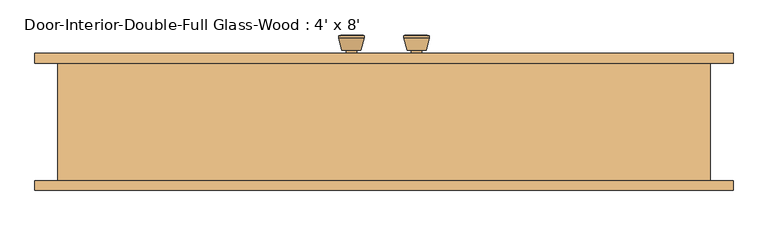
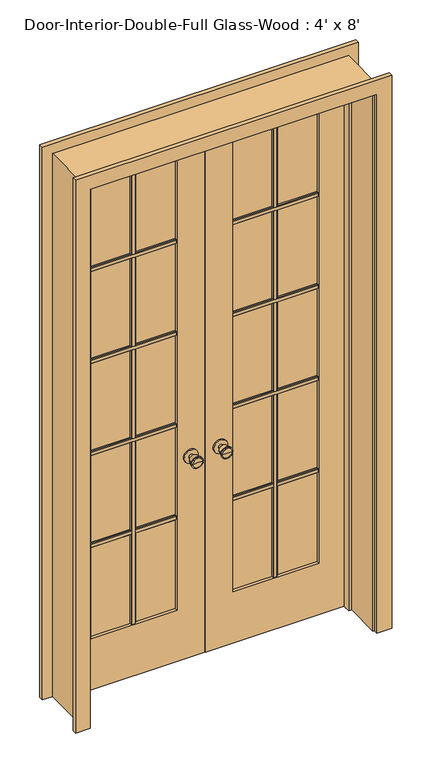
"""IFC4 building model written with IfcOpenShell, lengths in millimetres: door geometry, Door-Interior-Double-Full Glass-Wood : 4' x 8'."""

from ifc_helpers import new_model, si_unit, point, frame, frame_2d, origin, place, context, project, spatial, polyline, circle_curve, trimmed, segment, composite_curve, outline, extrude, faceted_brep, source, transform, mapped, element, save
from ifc_brep_helpers import plane_surface, cylinder_surface, revolved_surface, advanced_brep


def door_interior_double_full_glass_wood_4_x_8_0c92ad92(model_context):
    return source(origin(), model_context, "Body", "SolidModel", [
        advanced_brep(
        [(-63.5, 117.125, 914.4), (-73.5, 117.125, 914.4), (-53.5, 117.125, 914.4), (-83.9758676, 166.125, 914.4), (-63.5, 166.125, 914.4), (-43.0241324, 166.125, 914.4), (-88.5, 164.2971319, 914.4), (-38.5, 164.2971319, 914.4), (-88.5, 160.8334537, 914.4), (-38.5, 160.8334537, 914.4), (-82.136236, 136.125, 914.4), (-44.863764, 136.125, 914.4), (-73.5, 136.125, 914.4), (-53.5, 136.125, 914.4)],
        [
            (0, 1),
            (1, 2, circle_curve(frame((-63.5, 117.125, 914.4), z_axis=(0.0, -1.0, 0.0), x_axis=(1.0, 0.0, 0.0)), 10.0)),
            (2, 0),
            (2, 1, circle_curve(frame((-63.5, 117.125, 914.4), z_axis=(0.0, -1.0, 0.0), x_axis=(1.0, 0.0, 0.0)), 10.0)),
            (3, 4),
            (4, 5),
            (5, 3, circle_curve(frame((-63.5, 166.125, 914.4), z_axis=(0.0, 1.0, 0.0), x_axis=(1.0, 0.0, 0.0)), 20.4758676)),
            (3, 5, circle_curve(frame((-63.5, 166.125, 914.4), z_axis=(0.0, 1.0, 0.0), x_axis=(1.0, 0.0, 0.0)), 20.4758676)),
            (6, 3),
            (5, 7),
            (7, 6, circle_curve(frame((-63.5, 164.2971319, 914.4), z_axis=(0.0, 1.0, 0.0), x_axis=(1.0, 0.0, 0.0)), 25.0)),
            (6, 7, circle_curve(frame((-63.5, 164.2971319, 914.4), z_axis=(0.0, 1.0, 0.0), x_axis=(1.0, 0.0, 0.0)), 25.0)),
            (8, 6),
            (7, 9),
            (9, 8, circle_curve(frame((-63.5, 160.8334537, 914.4), z_axis=(0.0, 1.0, 0.0), x_axis=(1.0, 0.0, 0.0)), 25.0)),
            (8, 9, circle_curve(frame((-63.5, 160.8334537, 914.4), z_axis=(0.0, 1.0, 0.0), x_axis=(1.0, 0.0, 0.0)), 25.0)),
            (10, 8),
            (9, 11),
            (11, 10, circle_curve(frame((-63.5, 136.125, 914.4), z_axis=(0.0, 1.0, 0.0), x_axis=(1.0, 0.0, 0.0)), 18.636236)),
            (10, 11, circle_curve(frame((-63.5, 136.125, 914.4), z_axis=(0.0, 1.0, 0.0), x_axis=(1.0, 0.0, 0.0)), 18.636236)),
            (12, 10),
            (11, 13),
            (13, 12, circle_curve(frame((-63.5, 136.125, 914.4), z_axis=(0.0, 1.0, 0.0), x_axis=(1.0, 0.0, 0.0)), 10.0)),
            (12, 13, circle_curve(frame((-63.5, 136.125, 914.4), z_axis=(0.0, 1.0, 0.0), x_axis=(1.0, 0.0, 0.0)), 10.0)),
            (1, 12),
            (13, 2),
        ],
        [
            plane_surface(frame((-63.5, 117.125, 914.4), z_axis=(0.0, -1.0, 0.0), x_axis=(1.0, 0.0, 0.0))),
            plane_surface(frame((-63.5, 166.125, 914.4), z_axis=(0.0, 1.0, 0.0), x_axis=(1.0, 0.0, 0.0))),
            revolved_surface(polyline([(-43.0241324, 166.125, 914.4), (-38.5, 164.2971319, 914.4)]), (-63.5, 117.125, 914.4), (0.0, -1.0, 0.0)),
            cylinder_surface(frame((-63.5, 117.125, 914.4), z_axis=(0.0, -1.0, 0.0), x_axis=(1.0, 0.0, 0.0)), 25.0),
            revolved_surface(polyline([(-38.5, 160.8334537, 914.4), (-44.863764, 136.125, 914.4)]), (-63.5, 117.125, 914.4), (0.0, -1.0, 0.0)),
            plane_surface(frame((-63.5, 136.125, 914.4), z_axis=(0.0, -1.0, 0.0), x_axis=(1.0, 0.0, 0.0))),
            cylinder_surface(frame((-63.5, 117.125, 914.4), z_axis=(0.0, -1.0, 0.0), x_axis=(1.0, 0.0, 0.0)), 10.0),
        ],
        [
            (0, [[1, 2, 3]]),
            (0, [[-3, 4, -1]]),
            (1, [[5, 6, 7]]),
            (1, [[-6, -5, 8]]),
            (2, [[9, -7, 10, 11]]),
            (2, [[-10, -8, -9, 12]]),
            (3, [[13, -11, 14, 15]]),
            (3, [[-14, -12, -13, 16]]),
            (4, [[17, -15, 18, 19]]),
            (4, [[-18, -16, -17, 20]]),
            (5, [[21, -19, 22, 23]]),
            (5, [[-22, -20, -21, 24]]),
            (6, [[25, -23, 26, -2]]),
            (6, [[-26, -24, -25, -4]]),
        ],
    ),
        extrude(outline(composite_curve([segment(trimmed(circle_curve(frame_2d((914.4, -63.5)), 30.0), [point((914.4, -33.5))], [point((914.4, -93.5))], False, "CARTESIAN"), True, "CONTINUOUS"), segment(trimmed(circle_curve(frame_2d((914.4, -63.5)), 30.0), [point((914.4, -93.5))], [point((914.4, -33.5))], False, "CARTESIAN"), True, "CONTINUOUS")], self_intersect=False)), frame((0.0, 111.125, 0.0), z_axis=(0.0, 1.0, 0.0), x_axis=(0.0, 0.0, 1.0)), (0.0, 0.0, 1.0), 6.0),
        advanced_brep(
        [(-63.5, 70.2, 914.4), (-53.5, 70.2, 914.4), (-73.5, 70.2, 914.4), (-83.9758676, 21.2, 914.4), (-43.0241324, 21.2, 914.4), (-63.5, 21.2, 914.4), (-88.5, 23.0278681, 914.4), (-38.5, 23.0278681, 914.4), (-88.5, 26.4915463, 914.4), (-38.5, 26.4915463, 914.4), (-82.136236, 51.2, 914.4), (-44.863764, 51.2, 914.4), (-73.5, 51.2, 914.4), (-53.5, 51.2, 914.4)],
        [
            (0, 1),
            (1, 2, circle_curve(frame((-63.5, 70.2, 914.4), z_axis=(0.0, 1.0, 0.0), x_axis=(1.0, 0.0, 0.0)), 10.0)),
            (2, 0),
            (2, 1, circle_curve(frame((-63.5, 70.2, 914.4), z_axis=(0.0, 1.0, 0.0), x_axis=(1.0, 0.0, 0.0)), 10.0)),
            (3, 4, circle_curve(frame((-63.5, 21.2, 914.4), z_axis=(0.0, -1.0, 0.0), x_axis=(1.0, 0.0, 0.0)), 20.4758676)),
            (4, 5),
            (5, 3),
            (4, 3, circle_curve(frame((-63.5, 21.2, 914.4), z_axis=(0.0, -1.0, 0.0), x_axis=(1.0, 0.0, 0.0)), 20.4758676)),
            (6, 7, circle_curve(frame((-63.5, 23.0278681, 914.4), z_axis=(0.0, -1.0, 0.0), x_axis=(1.0, 0.0, 0.0)), 25.0)),
            (7, 4),
            (3, 6),
            (7, 6, circle_curve(frame((-63.5, 23.0278681, 914.4), z_axis=(0.0, -1.0, 0.0), x_axis=(1.0, 0.0, 0.0)), 25.0)),
            (8, 9, circle_curve(frame((-63.5, 26.4915463, 914.4), z_axis=(0.0, -1.0, 0.0), x_axis=(1.0, 0.0, 0.0)), 25.0)),
            (9, 7),
            (6, 8),
            (9, 8, circle_curve(frame((-63.5, 26.4915463, 914.4), z_axis=(0.0, -1.0, 0.0), x_axis=(1.0, 0.0, 0.0)), 25.0)),
            (10, 11, circle_curve(frame((-63.5, 51.2, 914.4), z_axis=(0.0, -1.0, 0.0), x_axis=(1.0, 0.0, 0.0)), 18.636236)),
            (11, 9),
            (8, 10),
            (11, 10, circle_curve(frame((-63.5, 51.2, 914.4), z_axis=(0.0, -1.0, 0.0), x_axis=(1.0, 0.0, 0.0)), 18.636236)),
            (12, 13, circle_curve(frame((-63.5, 51.2, 914.4), z_axis=(0.0, -1.0, 0.0), x_axis=(1.0, 0.0, 0.0)), 10.0)),
            (13, 11),
            (10, 12),
            (13, 12, circle_curve(frame((-63.5, 51.2, 914.4), z_axis=(0.0, -1.0, 0.0), x_axis=(1.0, 0.0, 0.0)), 10.0)),
            (1, 13),
            (12, 2),
        ],
        [
            plane_surface(frame((-63.5, 70.2, 914.4), z_axis=(0.0, 1.0, 0.0), x_axis=(1.0, 0.0, 0.0))),
            plane_surface(frame((-63.5, 21.2, 914.4), z_axis=(0.0, -1.0, 0.0), x_axis=(1.0, 0.0, 0.0))),
            revolved_surface(polyline([(-43.0241324, 21.2, 914.4), (-38.5, 23.0278681, 914.4)]), (-63.5, 70.2, 914.4), (0.0, 1.0, 0.0)),
            cylinder_surface(frame((-63.5, 70.2, 914.4), z_axis=(0.0, 1.0, 0.0), x_axis=(1.0, 0.0, 0.0)), 25.0),
            revolved_surface(polyline([(-38.5, 26.4915463, 914.4), (-44.863764, 51.2, 914.4)]), (-63.5, 70.2, 914.4), (0.0, 1.0, 0.0)),
            plane_surface(frame((-63.5, 51.2, 914.4), z_axis=(0.0, 1.0, 0.0), x_axis=(1.0, 0.0, 0.0))),
            cylinder_surface(frame((-63.5, 70.2, 914.4), z_axis=(0.0, 1.0, 0.0), x_axis=(1.0, 0.0, 0.0)), 10.0),
        ],
        [
            (0, [[1, 2, 3]]),
            (0, [[-3, 4, -1]]),
            (1, [[5, 6, 7]]),
            (1, [[8, -7, -6]]),
            (2, [[9, 10, -5, 11]]),
            (2, [[12, -11, -8, -10]]),
            (3, [[13, 14, -9, 15]]),
            (3, [[16, -15, -12, -14]]),
            (4, [[17, 18, -13, 19]]),
            (4, [[20, -19, -16, -18]]),
            (5, [[21, 22, -17, 23]]),
            (5, [[24, -23, -20, -22]]),
            (6, [[-2, 25, -21, 26]]),
            (6, [[-4, -26, -24, -25]]),
        ],
    ),
        extrude(outline(composite_curve([segment(trimmed(circle_curve(frame_2d((914.4, -63.5)), 30.0), [point((914.4, -33.5))], [point((914.4, -93.5))], False, "CARTESIAN"), True, "CONTINUOUS"), segment(trimmed(circle_curve(frame_2d((914.4, -63.5)), 30.0), [point((914.4, -93.5))], [point((914.4, -33.5))], False, "CARTESIAN"), True, "CONTINUOUS")], self_intersect=False)), frame((0.0, 70.2, 0.0), z_axis=(0.0, 1.0, 0.0), x_axis=(0.0, 0.0, 1.0)), (0.0, 0.0, 1.0), 6.0),
        extrude(outline(polyline([(90.17, 1911.35), (90.17, 1892.3), (83.82, 1892.3), (80.645, 1895.475), (80.645, 1908.175), (83.82, 1911.35), (90.17, 1911.35)])), frame((120.65, 0.0, 0.0), z_axis=(1.0, 0.0, 0.0), x_axis=(0.0, 1.0, 0.0)), (0.0, 0.0, 1.0), 368.3),
        extrude(outline(polyline([(90.17, 1493.8375), (90.17, 1474.7875), (83.82, 1474.7875), (80.645, 1477.9625), (80.645, 1490.6625), (83.82, 1493.8375), (90.17, 1493.8375)])), frame((120.65, 0.0, 0.0), z_axis=(1.0, 0.0, 0.0), x_axis=(0.0, 1.0, 0.0)), (0.0, 0.0, 1.0), 368.3),
        extrude(outline(polyline([(90.17, 1076.325), (90.17, 1057.275), (83.82, 1057.275), (80.645, 1060.45), (80.645, 1073.15), (83.82, 1076.325), (90.17, 1076.325)])), frame((120.65, 0.0, 0.0), z_axis=(1.0, 0.0, 0.0), x_axis=(0.0, 1.0, 0.0)), (0.0, 0.0, 1.0), 368.3),
        extrude(outline(polyline([(295.275, 90.17), (314.325, 90.17), (314.325, 83.82), (311.15, 80.645), (298.45, 80.645), (295.275, 83.82), (295.275, 90.17)])), frame((0.0, 0.0, 231.775), z_axis=(0.0, 0.0, 1.0), x_axis=(1.0, 0.0, 0.0)), (0.0, 0.0, 1.0), 2087.5625),
        extrude(outline(polyline([(90.17, 658.8125), (90.17, 639.7625), (83.82, 639.7625), (80.645, 642.9375), (80.645, 655.6375), (83.82, 658.8125), (90.17, 658.8125)])), frame((120.65, 0.0, 0.0), z_axis=(1.0, 0.0, 0.0), x_axis=(0.0, 1.0, 0.0)), (0.0, 0.0, 1.0), 368.3),
        extrude(outline(polyline([(97.155, 1911.35), (103.505, 1911.35), (106.68, 1908.175), (106.68, 1895.475), (103.505, 1892.3), (97.155, 1892.3), (97.155, 1911.35)])), frame((-488.95, 0.0, 0.0), z_axis=(1.0, 0.0, 0.0), x_axis=(0.0, 1.0, 0.0)), (0.0, 0.0, 1.0), 368.3),
        extrude(outline(polyline([(97.155, 1493.8375), (103.505, 1493.8375), (106.68, 1490.6625), (106.68, 1477.9625), (103.505, 1474.7875), (97.155, 1474.7875), (97.155, 1493.8375)])), frame((-488.95, 0.0, 0.0), z_axis=(1.0, 0.0, 0.0), x_axis=(0.0, 1.0, 0.0)), (0.0, 0.0, 1.0), 368.3),
        extrude(outline(polyline([(97.155, 1076.325), (103.505, 1076.325), (106.68, 1073.15), (106.68, 1060.45), (103.505, 1057.275), (97.155, 1057.275), (97.155, 1076.325)])), frame((-488.95, 0.0, 0.0), z_axis=(1.0, 0.0, 0.0), x_axis=(0.0, 1.0, 0.0)), (0.0, 0.0, 1.0), 368.3),
        extrude(outline(polyline([(-314.325, 97.155), (-314.325, 103.505), (-311.15, 106.68), (-298.45, 106.68), (-295.275, 103.505), (-295.275, 97.155), (-314.325, 97.155)])), frame((0.0, 0.0, 231.775), z_axis=(0.0, 0.0, 1.0), x_axis=(1.0, 0.0, 0.0)), (0.0, 0.0, 1.0), 2087.5625),
        extrude(outline(polyline([(97.155, 658.8125), (103.505, 658.8125), (106.68, 655.6375), (106.68, 642.9375), (103.505, 639.7625), (97.155, 639.7625), (97.155, 658.8125)])), frame((-488.95, 0.0, 0.0), z_axis=(1.0, 0.0, 0.0), x_axis=(0.0, 1.0, 0.0)), (0.0, 0.0, 1.0), 368.3),
        extrude(outline(polyline([(97.155, 1911.35), (103.505, 1911.35), (106.68, 1908.175), (106.68, 1895.475), (103.505, 1892.3), (97.155, 1892.3), (97.155, 1911.35)])), frame((120.65, 0.0, 0.0), z_axis=(1.0, 0.0, 0.0), x_axis=(0.0, 1.0, 0.0)), (0.0, 0.0, 1.0), 368.3),
        extrude(outline(polyline([(97.155, 1493.8375), (103.505, 1493.8375), (106.68, 1490.6625), (106.68, 1477.9625), (103.505, 1474.7875), (97.155, 1474.7875), (97.155, 1493.8375)])), frame((120.65, 0.0, 0.0), z_axis=(1.0, 0.0, 0.0), x_axis=(0.0, 1.0, 0.0)), (0.0, 0.0, 1.0), 368.3),
        extrude(outline(polyline([(97.155, 1076.325), (103.505, 1076.325), (106.68, 1073.15), (106.68, 1060.45), (103.505, 1057.275), (97.155, 1057.275), (97.155, 1076.325)])), frame((120.65, 0.0, 0.0), z_axis=(1.0, 0.0, 0.0), x_axis=(0.0, 1.0, 0.0)), (0.0, 0.0, 1.0), 368.3),
        extrude(outline(polyline([(295.275, 97.155), (295.275, 103.505), (298.45, 106.68), (311.15, 106.68), (314.325, 103.505), (314.325, 97.155), (295.275, 97.155)])), frame((0.0, 0.0, 231.775), z_axis=(0.0, 0.0, 1.0), x_axis=(1.0, 0.0, 0.0)), (0.0, 0.0, 1.0), 2087.5625),
        extrude(outline(polyline([(97.155, 658.8125), (103.505, 658.8125), (106.68, 655.6375), (106.68, 642.9375), (103.505, 639.7625), (97.155, 639.7625), (97.155, 658.8125)])), frame((120.65, 0.0, 0.0), z_axis=(1.0, 0.0, 0.0), x_axis=(0.0, 1.0, 0.0)), (0.0, 0.0, 1.0), 368.3),
        extrude(outline(polyline([(90.17, 1911.35), (90.17, 1892.3), (83.82, 1892.3), (80.645, 1895.475), (80.645, 1908.175), (83.82, 1911.35), (90.17, 1911.35)])), frame((-488.95, 0.0, 0.0), z_axis=(1.0, 0.0, 0.0), x_axis=(0.0, 1.0, 0.0)), (0.0, 0.0, 1.0), 368.3),
        extrude(outline(polyline([(90.17, 1493.8375), (90.17, 1474.7875), (83.82, 1474.7875), (80.645, 1477.9625), (80.645, 1490.6625), (83.82, 1493.8375), (90.17, 1493.8375)])), frame((-488.95, 0.0, 0.0), z_axis=(1.0, 0.0, 0.0), x_axis=(0.0, 1.0, 0.0)), (0.0, 0.0, 1.0), 368.3),
        extrude(outline(polyline([(90.17, 1076.325), (90.17, 1057.275), (83.82, 1057.275), (80.645, 1060.45), (80.645, 1073.15), (83.82, 1076.325), (90.17, 1076.325)])), frame((-488.95, 0.0, 0.0), z_axis=(1.0, 0.0, 0.0), x_axis=(0.0, 1.0, 0.0)), (0.0, 0.0, 1.0), 368.3),
        extrude(outline(polyline([(-314.325, 90.17), (-295.275, 90.17), (-295.275, 83.82), (-298.45, 80.645), (-311.15, 80.645), (-314.325, 83.82), (-314.325, 90.17)])), frame((0.0, 0.0, 231.775), z_axis=(0.0, 0.0, 1.0), x_axis=(1.0, 0.0, 0.0)), (0.0, 0.0, 1.0), 2087.5625),
        extrude(outline(polyline([(90.17, 658.8125), (90.17, 639.7625), (83.82, 639.7625), (80.645, 642.9375), (80.645, 655.6375), (83.82, 658.8125), (90.17, 658.8125)])), frame((-488.95, 0.0, 0.0), z_axis=(1.0, 0.0, 0.0), x_axis=(0.0, 1.0, 0.0)), (0.0, 0.0, 1.0), 368.3),
        advanced_brep(
        [(63.5, 70.2, 914.4), (73.5, 70.2, 914.4), (53.5, 70.2, 914.4), (83.9758676, 21.2, 914.4), (63.5, 21.2, 914.4), (43.0241324, 21.2, 914.4), (88.5, 23.0278681, 914.4), (38.5, 23.0278681, 914.4), (88.5, 26.4915463, 914.4), (38.5, 26.4915463, 914.4), (82.136236, 51.2, 914.4), (44.863764, 51.2, 914.4), (73.5, 51.2, 914.4), (53.5, 51.2, 914.4)],
        [
            (0, 1),
            (1, 2, circle_curve(frame((63.5, 70.2, 914.4), z_axis=(0.0, 1.0, 0.0), x_axis=(-1.0, 0.0, 0.0)), 10.0)),
            (2, 0),
            (2, 1, circle_curve(frame((63.5, 70.2, 914.4), z_axis=(0.0, 1.0, 0.0), x_axis=(-1.0, 0.0, 0.0)), 10.0)),
            (3, 4),
            (4, 5),
            (5, 3, circle_curve(frame((63.5, 21.2, 914.4), z_axis=(0.0, -1.0, 0.0), x_axis=(-1.0, 0.0, 0.0)), 20.4758676)),
            (3, 5, circle_curve(frame((63.5, 21.2, 914.4), z_axis=(0.0, -1.0, 0.0), x_axis=(-1.0, 0.0, 0.0)), 20.4758676)),
            (6, 3),
            (5, 7),
            (7, 6, circle_curve(frame((63.5, 23.0278681, 914.4), z_axis=(0.0, -1.0, 0.0), x_axis=(-1.0, 0.0, 0.0)), 25.0)),
            (6, 7, circle_curve(frame((63.5, 23.0278681, 914.4), z_axis=(0.0, -1.0, 0.0), x_axis=(-1.0, 0.0, 0.0)), 25.0)),
            (8, 6),
            (7, 9),
            (9, 8, circle_curve(frame((63.5, 26.4915463, 914.4), z_axis=(0.0, -1.0, 0.0), x_axis=(-1.0, 0.0, 0.0)), 25.0)),
            (8, 9, circle_curve(frame((63.5, 26.4915463, 914.4), z_axis=(0.0, -1.0, 0.0), x_axis=(-1.0, 0.0, 0.0)), 25.0)),
            (10, 8),
            (9, 11),
            (11, 10, circle_curve(frame((63.5, 51.2, 914.4), z_axis=(0.0, -1.0, 0.0), x_axis=(-1.0, 0.0, 0.0)), 18.636236)),
            (10, 11, circle_curve(frame((63.5, 51.2, 914.4), z_axis=(0.0, -1.0, 0.0), x_axis=(-1.0, 0.0, 0.0)), 18.636236)),
            (12, 10),
            (11, 13),
            (13, 12, circle_curve(frame((63.5, 51.2, 914.4), z_axis=(0.0, -1.0, 0.0), x_axis=(-1.0, 0.0, 0.0)), 10.0)),
            (12, 13, circle_curve(frame((63.5, 51.2, 914.4), z_axis=(0.0, -1.0, 0.0), x_axis=(-1.0, 0.0, 0.0)), 10.0)),
            (1, 12),
            (13, 2),
        ],
        [
            plane_surface(frame((63.5, 70.2, 914.4), z_axis=(0.0, 1.0, 0.0), x_axis=(-1.0, 0.0, 0.0))),
            plane_surface(frame((63.5, 21.2, 914.4), z_axis=(0.0, -1.0, 0.0), x_axis=(-1.0, 0.0, 0.0))),
            revolved_surface(polyline([(43.0241324, 21.2, 914.4), (38.5, 23.0278681, 914.4)]), (63.5, 70.2, 914.4), (0.0, 1.0, 0.0)),
            cylinder_surface(frame((63.5, 70.2, 914.4), z_axis=(0.0, 1.0, 0.0), x_axis=(-1.0, 0.0, 0.0)), 25.0),
            revolved_surface(polyline([(38.5, 26.4915463, 914.4), (44.863764, 51.2, 914.4)]), (63.5, 70.2, 914.4), (0.0, 1.0, 0.0)),
            plane_surface(frame((63.5, 51.2, 914.4), z_axis=(0.0, 1.0, 0.0), x_axis=(-1.0, 0.0, 0.0))),
            cylinder_surface(frame((63.5, 70.2, 914.4), z_axis=(0.0, 1.0, 0.0), x_axis=(-1.0, 0.0, 0.0)), 10.0),
        ],
        [
            (0, [[1, 2, 3]]),
            (0, [[-3, 4, -1]]),
            (1, [[5, 6, 7]]),
            (1, [[-6, -5, 8]]),
            (2, [[9, -7, 10, 11]]),
            (2, [[-10, -8, -9, 12]]),
            (3, [[13, -11, 14, 15]]),
            (3, [[-14, -12, -13, 16]]),
            (4, [[17, -15, 18, 19]]),
            (4, [[-18, -16, -17, 20]]),
            (5, [[21, -19, 22, 23]]),
            (5, [[-22, -20, -21, 24]]),
            (6, [[25, -23, 26, -2]]),
            (6, [[-26, -24, -25, -4]]),
        ],
    ),
        extrude(outline(composite_curve([segment(trimmed(circle_curve(frame_2d((914.4, 63.5)), 30.0), [point((914.4, 33.5))], [point((914.4, 93.5))], False, "CARTESIAN"), True, "CONTINUOUS"), segment(trimmed(circle_curve(frame_2d((914.4, 63.5)), 30.0), [point((914.4, 93.5))], [point((914.4, 33.5))], False, "CARTESIAN"), True, "CONTINUOUS")], self_intersect=False)), frame((0.0, 70.2, 0.0), z_axis=(0.0, 1.0, 0.0), x_axis=(0.0, 0.0, 1.0)), (0.0, 0.0, 1.0), 6.0),
        advanced_brep(
        [(63.5, 117.125, 914.4), (53.5, 117.125, 914.4), (73.5, 117.125, 914.4), (83.9758676, 166.125, 914.4), (43.0241324, 166.125, 914.4), (63.5, 166.125, 914.4), (88.5, 164.2971319, 914.4), (38.5, 164.2971319, 914.4), (88.5, 160.8334537, 914.4), (38.5, 160.8334537, 914.4), (82.136236, 136.125, 914.4), (44.863764, 136.125, 914.4), (73.5, 136.125, 914.4), (53.5, 136.125, 914.4)],
        [
            (0, 1),
            (1, 2, circle_curve(frame((63.5, 117.125, 914.4), z_axis=(0.0, -1.0, 0.0), x_axis=(-1.0, 0.0, 0.0)), 10.0)),
            (2, 0),
            (2, 1, circle_curve(frame((63.5, 117.125, 914.4), z_axis=(0.0, -1.0, 0.0), x_axis=(-1.0, 0.0, 0.0)), 10.0)),
            (3, 4, circle_curve(frame((63.5, 166.125, 914.4), z_axis=(0.0, 1.0, 0.0), x_axis=(-1.0, 0.0, 0.0)), 20.4758676)),
            (4, 5),
            (5, 3),
            (4, 3, circle_curve(frame((63.5, 166.125, 914.4), z_axis=(0.0, 1.0, 0.0), x_axis=(-1.0, 0.0, 0.0)), 20.4758676)),
            (6, 7, circle_curve(frame((63.5, 164.2971319, 914.4), z_axis=(0.0, 1.0, 0.0), x_axis=(-1.0, 0.0, 0.0)), 25.0)),
            (7, 4),
            (3, 6),
            (7, 6, circle_curve(frame((63.5, 164.2971319, 914.4), z_axis=(0.0, 1.0, 0.0), x_axis=(-1.0, 0.0, 0.0)), 25.0)),
            (8, 9, circle_curve(frame((63.5, 160.8334537, 914.4), z_axis=(0.0, 1.0, 0.0), x_axis=(-1.0, 0.0, 0.0)), 25.0)),
            (9, 7),
            (6, 8),
            (9, 8, circle_curve(frame((63.5, 160.8334537, 914.4), z_axis=(0.0, 1.0, 0.0), x_axis=(-1.0, 0.0, 0.0)), 25.0)),
            (10, 11, circle_curve(frame((63.5, 136.125, 914.4), z_axis=(0.0, 1.0, 0.0), x_axis=(-1.0, 0.0, 0.0)), 18.636236)),
            (11, 9),
            (8, 10),
            (11, 10, circle_curve(frame((63.5, 136.125, 914.4), z_axis=(0.0, 1.0, 0.0), x_axis=(-1.0, 0.0, 0.0)), 18.636236)),
            (12, 13, circle_curve(frame((63.5, 136.125, 914.4), z_axis=(0.0, 1.0, 0.0), x_axis=(-1.0, 0.0, 0.0)), 10.0)),
            (13, 11),
            (10, 12),
            (13, 12, circle_curve(frame((63.5, 136.125, 914.4), z_axis=(0.0, 1.0, 0.0), x_axis=(-1.0, 0.0, 0.0)), 10.0)),
            (1, 13),
            (12, 2),
        ],
        [
            plane_surface(frame((63.5, 117.125, 914.4), z_axis=(0.0, -1.0, 0.0), x_axis=(-1.0, 0.0, 0.0))),
            plane_surface(frame((63.5, 166.125, 914.4), z_axis=(0.0, 1.0, 0.0), x_axis=(-1.0, 0.0, 0.0))),
            revolved_surface(polyline([(43.0241324, 166.125, 914.4), (38.5, 164.2971319, 914.4)]), (63.5, 117.125, 914.4), (0.0, -1.0, 0.0)),
            cylinder_surface(frame((63.5, 117.125, 914.4), z_axis=(0.0, -1.0, 0.0), x_axis=(-1.0, 0.0, 0.0)), 25.0),
            revolved_surface(polyline([(38.5, 160.8334537, 914.4), (44.863764, 136.125, 914.4)]), (63.5, 117.125, 914.4), (0.0, -1.0, 0.0)),
            plane_surface(frame((63.5, 136.125, 914.4), z_axis=(0.0, -1.0, 0.0), x_axis=(-1.0, 0.0, 0.0))),
            cylinder_surface(frame((63.5, 117.125, 914.4), z_axis=(0.0, -1.0, 0.0), x_axis=(-1.0, 0.0, 0.0)), 10.0),
        ],
        [
            (0, [[1, 2, 3]]),
            (0, [[-3, 4, -1]]),
            (1, [[5, 6, 7]]),
            (1, [[8, -7, -6]]),
            (2, [[9, 10, -5, 11]]),
            (2, [[12, -11, -8, -10]]),
            (3, [[13, 14, -9, 15]]),
            (3, [[16, -15, -12, -14]]),
            (4, [[17, 18, -13, 19]]),
            (4, [[20, -19, -16, -18]]),
            (5, [[21, 22, -17, 23]]),
            (5, [[24, -23, -20, -22]]),
            (6, [[-2, 25, -21, 26]]),
            (6, [[-4, -26, -24, -25]]),
        ],
    ),
        extrude(outline(composite_curve([segment(trimmed(circle_curve(frame_2d((914.4, 63.5)), 30.0), [point((914.4, 33.5))], [point((914.4, 93.5))], False, "CARTESIAN"), True, "CONTINUOUS"), segment(trimmed(circle_curve(frame_2d((914.4, 63.5)), 30.0), [point((914.4, 93.5))], [point((914.4, 33.5))], False, "CARTESIAN"), True, "CONTINUOUS")], self_intersect=False)), frame((0.0, 111.125, 0.0), z_axis=(0.0, 1.0, 0.0), x_axis=(0.0, 0.0, 1.0)), (0.0, 0.0, 1.0), 6.0),
        extrude(outline(polyline([(0.0, 615.95), (0.0, 679.45), (2508.25, 679.45), (2508.25, -679.45), (0.0, -679.45), (0.0, -615.95), (2444.75, -615.95), (2444.75, 615.95), (0.0, 615.95)])), frame((0.0, -136.525, 0.0), z_axis=(0.0, 1.0, 0.0), x_axis=(0.0, 0.0, 1.0)), (0.0, 0.0, 1.0), 19.05),
        extrude(outline(polyline([(0.0, 615.95), (0.0, 679.45), (2508.25, 679.45), (2508.25, -679.45), (0.0, -679.45), (0.0, -615.95), (2444.75, -615.95), (2444.75, 615.95), (0.0, 615.95)])), frame((0.0, 111.125, 0.0), z_axis=(0.0, 1.0, 0.0), x_axis=(0.0, 0.0, 1.0)), (0.0, 0.0, 1.0), 19.05),
        faceted_brep([(635.0, 111.125, 0.0), (635.0, -117.475, 0.0), (609.6, -117.475, 0.0), (609.6, 41.275, 0.0), (596.9, 41.275, 0.0), (596.9, 76.2, 0.0), (609.6, 76.2, 0.0), (609.6, 111.125, 0.0), (635.0, 111.125, 2463.8), (635.0, -117.475, 2463.8), (-635.0, -117.475, 2463.8), (-635.0, -117.475, 0.0), (-609.6, -117.475, 0.0), (-609.6, -117.475, 2438.4), (609.6, -117.475, 2438.4), (609.6, 41.275, 2438.4), (-609.6, 41.275, 2438.4), (-609.6, 41.275, 0.0), (-596.9, 41.275, 0.0), (-596.9, 41.275, 2425.7), (596.9, 41.275, 2425.7), (596.9, 76.2, 2425.7), (1.5875, 76.2, 2425.7), (-1.6019111, 76.2, 2425.7), (-596.9, 76.2, 2425.7), (-596.9, 76.2, 0.0), (-609.6, 76.2, 0.0), (-609.6, 76.2, 2438.4), (-1.6019111, 76.2, 2438.4), (1.5875, 76.2, 2438.4), (609.6, 76.2, 2438.4), (609.6, 111.125, 2438.4), (1.5875, 111.125, 2438.4), (-1.6019111, 111.125, 2438.4), (-609.6, 111.125, 2438.4), (-609.6, 111.125, 0.0), (-635.0, 111.125, 0.0), (-635.0, 111.125, 2463.8)], [[[0, 1, 2, 3, 4, 5, 6, 7]], [[1, 0, 8, 9]], [[2, 1, 9, 10, 11, 12, 13, 14]], [[3, 2, 14, 15]], [[4, 3, 15, 16, 17, 18, 19, 20]], [[5, 4, 20, 21]], [[6, 5, 21, 22, 23, 24, 25, 26, 27, 28, 29, 30]], [[7, 6, 30, 31]], [[0, 7, 31, 32, 33, 34, 35, 36, 37, 8]], [[9, 8, 37, 10]], [[14, 13, 16, 15]], [[20, 19, 24, 23, 22, 21]], [[31, 30, 29, 28, 27, 34, 33, 32]], [[12, 11, 36, 35, 26, 25, 18, 17]], [[11, 10, 37, 36]], [[13, 12, 17, 16]], [[19, 18, 25, 24]], [[27, 26, 35, 34]]]),
        extrude(outline(polyline([(2438.4, -609.6), (0.0, -609.6), (0.0, -1.6019111), (2438.4, -1.6019111), (2438.4, -609.6)]), holes=[polyline([(231.775, -488.95), (2319.3375, -488.95), (2319.3375, -120.65), (231.775, -120.65), (231.775, -488.95)])]), frame((0.0, 76.2, 0.0), z_axis=(0.0, 1.0, 0.0), x_axis=(0.0, 0.0, 1.0)), (0.0, 0.0, 1.0), 34.925),
        extrude(outline(polyline([(0.0, 609.6), (2438.4, 609.6), (2438.4, 1.5875), (0.0, 1.5875), (0.0, 609.6)]), holes=[polyline([(2319.3375, 120.65), (2319.3375, 488.95), (231.775, 488.95), (231.775, 120.65), (2319.3375, 120.65)])]), frame((0.0, 76.2, 0.0), z_axis=(0.0, 1.0, 0.0), x_axis=(0.0, 0.0, 1.0)), (0.0, 0.0, 1.0), 34.925),
        extrude(outline(polyline([(488.95, 90.17), (120.65, 90.17), (120.65, 97.155), (488.95, 97.155), (488.95, 90.17)])), frame((0.0, 0.0, 231.775), z_axis=(0.0, 0.0, 1.0), x_axis=(1.0, 0.0, 0.0)), (0.0, 0.0, 1.0), 2087.5625),
        extrude(outline(polyline([(-120.65, 90.17), (-488.95, 90.17), (-488.95, 97.155), (-120.65, 97.155), (-120.65, 90.17)])), frame((0.0, 0.0, 231.775), z_axis=(0.0, 0.0, 1.0), x_axis=(1.0, 0.0, 0.0)), (0.0, 0.0, 1.0), 2087.5625),
    ])


if __name__ == "__main__":
    model = new_model("IFC4")
    model_context = context("Model", 3, world=origin())
    ifc_project = project(units=[si_unit("LENGTHUNIT", "METRE", prefix="MILLI")], contexts=[model_context])
    site = spatial("IfcSite", under=ifc_project)
    building = spatial("IfcBuilding", under=site)
    placement = place(None, origin())
    door_interior_double_full_glass_wood_4_x_8_shape = door_interior_double_full_glass_wood_4_x_8_0c92ad92(model_context)
    element("IfcDoor", 1, ObjectType="Door-Interior-Double-Full Glass-Wood : 4' x 8'", at=placement, inside=building, context=model_context, shape_type="MappedRepresentation", body=[
        mapped(door_interior_double_full_glass_wood_4_x_8_shape, transform((0.0, 0.0, 0.0), x_axis=(1.0, 0.0, 0.0), y_axis=(0.0, 1.0, 0.0), z_axis=(0.0, 0.0, 1.0))),
    ])
    save(model, "model.ifc")

# Revit data of these elements
# Type "Door-Interior-Double-Full Glass-Wood : 4' x 8'"
#   Type Mark = "11"
#   Assembly Code = "C1020300"
#   Analytic Construction = "French door, wood frame with single glass"
#   Top Rail = 0' - 4 11/16"
#   Thickness = 0' - 1 3/8"
#   Thermal Resistance (R) = 1.0696 (h·ft²·°F)/BTU
#   Swing Angle [instance default] = 90.00°
#   Stiles = 0' - 4 3/4"
#   Rough Width = 4' - 2"
#   Rough Height = 8' - 1"
#   Panel Width = 2' - 0"
#   Height = 8' - 0"
#   Width = 4' - 0"
#   Heat Transfer Coefficient (U) = 0.9350 BTU/(h·ft²·°F)
#   Bottom Rail = 0' - 9 1/8"
#   Show Grill [instance default] = yes
#   Trim Material = Cherry
#   Panel Material = Cherry
#   Frame Material = Cherry
#   Door Handle Material = Aluminum
#   Visual Light Transmittance = 0
#   Solar Heat Gain Coefficient = 0
#   Wall Closure = (empty or 0)
#   Function = (empty or 0)
# Element 1 (IfcDoor, "Door-Interior-Double-Full Glass-Wood : 4' x 8'")
#   Materials on its faces: "Cherry", "Aluminum", "Glass"
# Materials
#   "Cherry": class "Wood", colour RGB 226 177 128, transparency 0, Description = "Prunus Serotina", Cost = 0
#   "Aluminum": class "Metal", colour RGB 247 247 247, transparency 0, Description = "Aluminum 6061", Cost = 0
#   "Glass": class "Glass", colour RGB 0 128 192, transparency 0.75, Description = "Soda Lime Glass", Cost = 0
